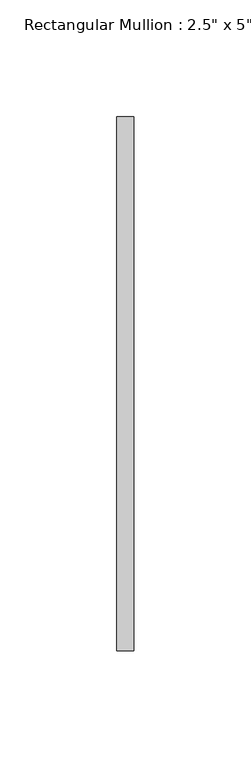
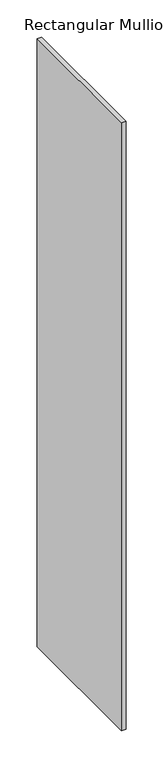
"""IFC4 building model written with IfcOpenShell, lengths in millimetres: member geometry."""

from ifc_helpers import new_model, si_unit, frame, origin, place, context, project, spatial, polyline, outline, extrude, source, transform, mapped, element, save


def member_1c5a217c(model_context):
    return source(origin(), model_context, "Body", "SweptSolid", [
        extrude(outline(polyline([(3.6195, 114.3), (3.6195, -114.3), (-3.6195, -114.3), (-3.6195, 114.3), (3.6195, 114.3)])), frame((0.0, 0.0, -1003.3), z_axis=(0.0, 0.0, 1.0), x_axis=(1.0, 0.0, 0.0)), (0.0, 0.0, 1.0), 1003.3),
    ])


if __name__ == "__main__":
    model = new_model("IFC4")
    model_context = context("Model", 3, world=origin())
    ifc_project = project(units=[si_unit("LENGTHUNIT", "METRE", prefix="MILLI")], contexts=[model_context])
    site = spatial("IfcSite", under=ifc_project)
    building = spatial("IfcBuilding", under=site)
    placement = place(None, origin())
    member_shape = member_1c5a217c(model_context)
    element("IfcMember", 1, ObjectType="Rectangular Mullion : 2.5\" x 5\" rectangular", at=placement, inside=building, context=model_context, shape_type="MappedRepresentation", body=[
        mapped(member_shape, transform((0.0, 0.0, 0.0), x_axis=(1.0, 0.0, 0.0), y_axis=(0.0, 1.0, 0.0), z_axis=(0.0, 0.0, 1.0))),
    ])
    save(model, "model.ifc")

# Revit data of these elements
# Type "Rectangular Mullion : 2.5\" x 5\" rectangular"
#   built-in parameter 1007304 = 0.75 (stored number, unit not read)
#   built-in parameter 1007301 = 0.011875 (stored number, unit not read)
#   built-in parameter 1007300 = 0.011875 (stored number, unit not read)
# Element 1 (IfcMember, "Rectangular Mullion : 2.5\" x 5\" rectangular")
#   Materials on its faces: "WINDOW GLASS MATERIAL"
# Materials
#   "WINDOW GLASS MATERIAL": class "Generic", colour RGB 120 120 120, transparency 0, Cost = 0
